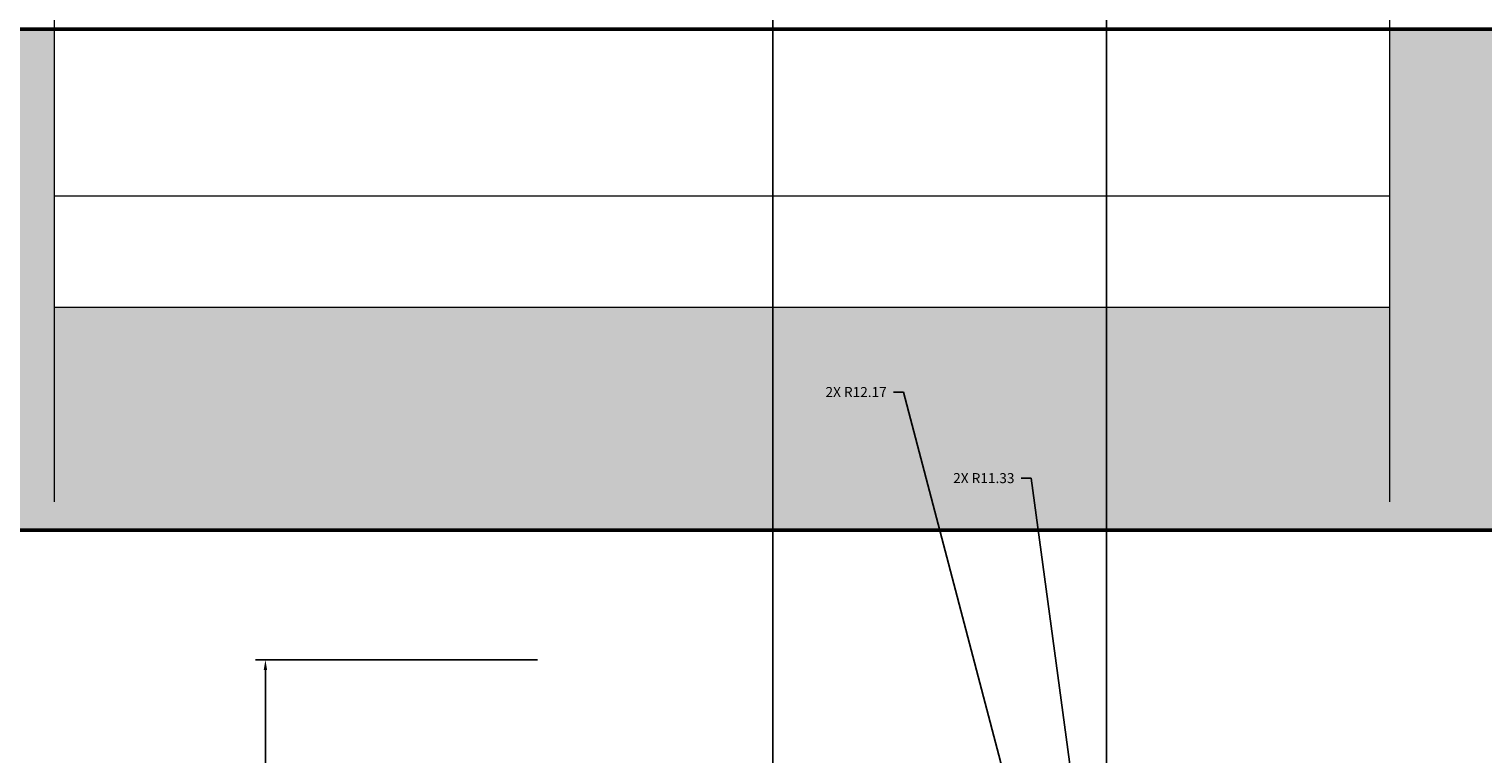
# Model space of a CAD drawing. Units: inches. Extents: x 2307 to 2544, y 2171 to 2540.
# Tile 47 of 52: x 2472 to 2498, y 2507 to 2521. Entities that reach past the tile are written whole.
import ezdxf

# ---------------------------------------------------------------- set-up
doc = ezdxf.new("R2010")
doc.units = ezdxf.units.IN
for name, color, linetype, lineweight in [('A-ANNO-DIMS', 2, 'Continuous', 18), ('A-GLAZ', 4, 'Continuous', 18), ('A-WALL', 7, 'Continuous', 50)]:
    doc.layers.add(name, color=color, linetype=linetype, lineweight=lineweight)
doc.layers.add('A-WALL-PATT', color=18, linetype='Continuous', lineweight=13, true_color=0x000000)
doc.styles.get("Standard").update_dxf_attribs({"font": 'arial.ttf'})
doc.dimstyles.get("Standard").update_dxf_attribs({"dimtxt": 0.18, "dimasz": 0.18, "dimexe": 0.18, "dimexo": 0.0625, "dimgap": 0.09, "dimtad": 0, "dimtih": 1, "dimtoh": 1, "dimdec": 4, "dimzin": 0, "dimdsep": 46, "dimtxsty": 'Standard', "dimcen": 0.09, "dimadec": 0, "dimazin": 0, "dimtfac": 1, "dimtdec": 4, "dimtofl": 0, "dimtmove": 0, "dimatfit": 3, "dimfxl": 1, "dimtolj": 1, "dimtzin": 0, "dimarcsym": 0})

# ---------------------------------------------------------------- blocks, each defined once
blk = doc.blocks.new('*D21')
at = {"layer": 'A-ANNO-DIMS', "color": 0, "lineweight": -2, "transparency": 16777216}
for p, q in [((2481.469, 2509.177), (2476.395, 2509.177)), ((2476.575, 2508.997), (2476.575, 2498.858)), ((2476.575, 2488.357), (2476.575, 2498.497)), ((2481.469, 2488.177), (2476.395, 2488.177))]:
    blk.add_line(p, q, dxfattribs=at)
at = {"layer": 'A-ANNO-DIMS', "color": 0, "transparency": 16777216}
for points in [[(2476.545, 2508.997), (2476.605, 2508.997), (2476.575, 2509.177)], [(2476.545, 2488.357), (2476.605, 2488.357), (2476.575, 2488.177)]]:
    blk.add_solid(points, dxfattribs=at)
at = {"layer": 'Defpoints', "color": 0, "transparency": 16777216}
for p in [(2481.532, 2509.177), (2476.575, 2488.177), (2481.532, 2488.177)]:
    blk.add_point(p, dxfattribs=at)
at = {"layer": 'A-ANNO-DIMS', "color": 0, "transparency": 16777216, "insert": (2476.575, 2498.677), "char_height": 0.18, "attachment_point": 5}
blk.add_mtext('\\A1;21', dxfattribs=at)
blk = doc.blocks.new('*D46')
at = {"layer": 'A-ANNO-DIMS', "color": 0, "lineweight": -2, "transparency": 16777216}
for p, q in [((2455.696, 2511.572), (2455.696, 2540.345)), ((2515.696, 2511.572), (2515.696, 2540.345)), ((2455.876, 2540.165), (2485.477, 2540.165)), ((2515.516, 2540.165), (2485.915, 2540.165))]:
    blk.add_line(p, q, dxfattribs=at)
at = {"layer": 'A-ANNO-DIMS', "color": 0, "transparency": 16777216}
for points in [[(2455.876, 2540.195), (2455.876, 2540.135), (2455.696, 2540.165)], [(2515.516, 2540.195), (2515.516, 2540.135), (2515.696, 2540.165)]]:
    blk.add_solid(points, dxfattribs=at)
at = {"layer": 'Defpoints', "color": 0, "transparency": 16777216}
for p in [(2515.696, 2540.165), (2455.696, 2511.51), (2515.696, 2511.51)]:
    blk.add_point(p, dxfattribs=at)
at = {"layer": 'A-ANNO-DIMS', "color": 0, "transparency": 16777216, "insert": (2485.696, 2540.165), "char_height": 0.18, "attachment_point": 5}
blk.add_mtext('\\A1;60', dxfattribs=at)
blk = doc.blocks.new('*D59')
at = {"layer": 'A-ANNO-DIMS', "color": 0, "lineweight": -2, "transparency": 16777216}
for p, q in [((2455.696, 2315.572), (2455.696, 2540.345)), ((2485.696, 2315.572), (2485.696, 2540.345)), ((2455.876, 2540.165), (2470.477, 2540.165)), ((2485.516, 2540.165), (2470.914, 2540.165))]:
    blk.add_line(p, q, dxfattribs=at)
at = {"layer": 'A-ANNO-DIMS', "color": 0, "transparency": 16777216}
for points in [[(2455.876, 2540.195), (2455.876, 2540.135), (2455.696, 2540.165)], [(2485.516, 2540.195), (2485.516, 2540.135), (2485.696, 2540.165)]]:
    blk.add_solid(points, dxfattribs=at)
at = {"layer": 'Defpoints', "color": 0, "transparency": 16777216}
for p in [(2455.696, 2540.165), (2455.696, 2315.51), (2485.696, 2315.51)]:
    blk.add_point(p, dxfattribs=at)
at = {"layer": 'A-ANNO-DIMS', "color": 0, "transparency": 16777216, "insert": (2470.696, 2540.165), "char_height": 0.18, "attachment_point": 5}
blk.add_mtext('\\A1;30', dxfattribs=at)
blk = doc.blocks.new('*D61')
at = {"layer": 'A-ANNO-DIMS', "color": 0, "lineweight": -2, "transparency": 16777216}
for p, q in [((2491.696, 2435.572), (2491.696, 2540.345)), ((2515.696, 2435.572), (2515.696, 2540.345)), ((2491.876, 2540.165), (2503.476, 2540.165)), ((2515.516, 2540.165), (2503.916, 2540.165))]:
    blk.add_line(p, q, dxfattribs=at)
at = {"layer": 'A-ANNO-DIMS', "color": 0, "transparency": 16777216}
for points in [[(2491.876, 2540.195), (2491.876, 2540.135), (2491.696, 2540.165)], [(2515.516, 2540.195), (2515.516, 2540.135), (2515.696, 2540.165)]]:
    blk.add_solid(points, dxfattribs=at)
at = {"layer": 'Defpoints', "color": 0, "transparency": 16777216}
for p in [(2515.696, 2540.165), (2491.696, 2435.51), (2515.696, 2435.51)]:
    blk.add_point(p, dxfattribs=at)
at = {"layer": 'A-ANNO-DIMS', "color": 0, "transparency": 16777216, "insert": (2503.696, 2540.165), "char_height": 0.18, "attachment_point": 5}
blk.add_mtext('\\A1;24', dxfattribs=at)
blk = doc.blocks.new('*D71')
at = {"layer": 'A-ANNO-DIMS', "color": 0, "lineweight": -2, "transparency": 16777216}
for p, q in [((2487.87, 2513.989), (2488.05, 2513.989)), ((2488.05, 2513.989), (2489.859, 2507.101)), ((2492.997, 2495.068), (2492.997, 2495.248)), ((2492.907, 2495.158), (2493.087, 2495.158))]:
    blk.add_line(p, q, dxfattribs=at)
at = {"layer": 'A-ANNO-DIMS', "color": 0, "transparency": 16777216}
blk.add_solid([(2489.888, 2507.109), (2489.83, 2507.094), (2489.905, 2506.927)], dxfattribs=at)
at = {"layer": 'Defpoints', "color": 0, "transparency": 16777216}
for p in [(2489.905, 2506.927), (2492.997, 2495.158)]:
    blk.add_point(p, dxfattribs=at)
at = {"layer": 'A-ANNO-DIMS', "color": 0, "transparency": 16777216, "insert": (2487.195, 2513.989), "char_height": 0.18, "attachment_point": 5}
blk.add_mtext('\\A1;2X R12.17', dxfattribs=at)
blk = doc.blocks.new('*D72')
at = {"layer": 'A-ANNO-DIMS', "color": 0, "lineweight": -2, "transparency": 16777216}
for p, q in [((2490.165, 2512.442), (2490.345, 2512.442)), ((2490.345, 2512.442), (2491.227, 2505.884)), ((2492.67, 2494.477), (2492.85, 2494.477)), ((2492.76, 2494.387), (2492.76, 2494.567))]:
    blk.add_line(p, q, dxfattribs=at)
at = {"layer": 'A-ANNO-DIMS', "color": 0, "transparency": 16777216}
blk.add_solid([(2491.257, 2505.888), (2491.197, 2505.88), (2491.251, 2505.705)], dxfattribs=at)
at = {"layer": 'Defpoints', "color": 0, "transparency": 16777216}
for p in [(2491.251, 2505.705), (2492.76, 2494.477)]:
    blk.add_point(p, dxfattribs=at)
at = {"layer": 'A-ANNO-DIMS', "color": 0, "transparency": 16777216, "insert": (2489.491, 2512.442), "char_height": 0.18, "attachment_point": 5}
blk.add_mtext('\\A1;2X R11.33', dxfattribs=at)

msp = doc.modelspace()

# ---------------------------------------------------------------- hatches: boundary and pattern name
at = {"layer": 'A-WALL-PATT'}
h = msp.add_hatch(color=256, dxfattribs=at)
h.dxf.hatch_style = 1
h.paths.add_polyline_path([(2433.6935, 2199.5096), (2415.6423, 2199.5096), (2415.6423, 2190.5096), (2433.7832, 2190.5096)], flags=17)
h.paths.add_polyline_path([(2367.6423, 2199.5096), (2335.6958, 2199.5096), (2335.6958, 2307.3983), (2326.6958, 2307.3983), (2326.6958, 2190.5096), (2367.6423, 2190.5096)])
h.paths.add_polyline_path([(2524.6958, 2520.5096), (2496.7832, 2520.5096), (2496.7832, 2515.5149), (2472.7832, 2515.5149), (2472.7832, 2520.5096), (2415.4028, 2520.5096), (2415.4028, 2511.5096), (2451.6958, 2511.5096), (2451.6958, 2439.5096), (2451.6958, 2391.5096), (2445.6958, 2391.5096), (2445.6958, 2387.5096), (2455.6958, 2387.5096), (2455.6958, 2435.5096), (2461.6958, 2435.5096), (2461.6958, 2439.5096), (2455.6958, 2439.5096), (2455.6958, 2511.5096), (2515.6958, 2511.5096), (2515.6958, 2439.5096), (2491.6958, 2439.5096), (2491.6958, 2435.5096), (2515.6958, 2435.5096), (2515.6958, 2319.5096), (2451.6958, 2319.5096), (2451.6958, 2281.5096), (2481.6958, 2281.5096), (2481.6958, 2225.5096), (2485.6958, 2225.5096), (2485.6958, 2285.5096), (2455.6958, 2285.5096), (2455.6958, 2315.5096), (2515.6958, 2315.5096), (2515.6958, 2199.5096), (2469.6952, 2199.5096), (2469.785, 2190.5096), (2524.6958, 2190.5096)])

# ---------------------------------------------------------------- linework, layer by layer
at = {"layer": 'A-GLAZ'}
for p, q in [((2472.7832, 2517.5149), (2496.7832, 2517.5149)), ((2472.7832, 2515.5149), (2496.7832, 2515.5149))]:
    msp.add_line(p, q, dxfattribs=at)
for points in [[(2472.7832, 2512.0149), (2472.7832, 2521.0149)], [(2496.7832, 2521.0149), (2496.7832, 2512.0149)]]:
    msp.add_lwpolyline(points, dxfattribs=at)
at = {"layer": 'A-WALL'}
msp.add_line((2455.6958, 2511.5096), (2515.6958, 2511.5096), dxfattribs=at)
msp.add_lwpolyline([(2433.7832, 2190.5096), (2326.6958, 2190.5096), (2326.6958, 2520.5096), (2524.6958, 2520.5096), (2524.6958, 2190.5096), (2469.785, 2190.5096)], dxfattribs=at)

# ---------------------------------------------------------------- dimensions: what is measured, and where the dimension line sits
at = {"layer": 'A-ANNO-DIMS'}
for base, p1, p2, picture, middle in [((2515.6958, 2540.1649), (2455.6958, 2511.5096), (2515.6958, 2511.5096), '*D46', (2485.6958, 2540.1649)), ((2455.6958, 2540.1649), (2485.6958, 2315.5096), (2455.6958, 2315.5096), '*D59', (2470.6958, 2540.1649)), ((2515.6958, 2540.1649), (2491.6958, 2435.5096), (2515.6958, 2435.5096), '*D61', (2503.6958, 2540.1649))]:
    dim = msp.add_linear_dim(base=base, p1=p1, p2=p2, dimstyle='Standard', override={"dimdec": 0, "dimlfac": 1, "dimrnd": 0, "dimzin": 0, "dimdsep": 46, "dimlunit": 2}, dxfattribs=at)
    dim.commit()
    dim.dimension.update_dxf_attribs({"geometry": picture, "text_midpoint": middle})
for center, mpoint, picture, middle in [((2492.9973, 2495.1576), (2489.905, 2506.9272), '*D71', (2487.1948, 2513.9889)), ((2492.7604, 2494.4772), (2491.2509, 2505.7054), '*D72', (2489.4905, 2512.4423))]:
    dim = msp.add_radius_dim(center=center, mpoint=mpoint, text='2X <>', dimstyle='Standard', override={"dimdec": 2, "dimlfac": 1, "dimrnd": 0, "dimzin": 0, "dimdsep": 46, "dimlunit": 2}, dxfattribs=at)
    dim.commit()
    dim.dimension.update_dxf_attribs({"geometry": picture, "text_midpoint": middle, "dimtype": 164})
dim = msp.add_linear_dim(base=(2476.5746, 2488.1772), p1=(2481.5315, 2509.1772), p2=(2481.5315, 2488.1772), angle=270, dimstyle='Standard', override={"dimdec": 0, "dimlfac": 1, "dimrnd": 0, "dimzin": 0, "dimdsep": 46, "dimlunit": 2}, dxfattribs=at)
dim.commit()
dim.dimension.update_dxf_attribs({"geometry": '*D21', "text_midpoint": (2476.5746, 2498.6772)})

doc.saveas('drawing.dxf')
